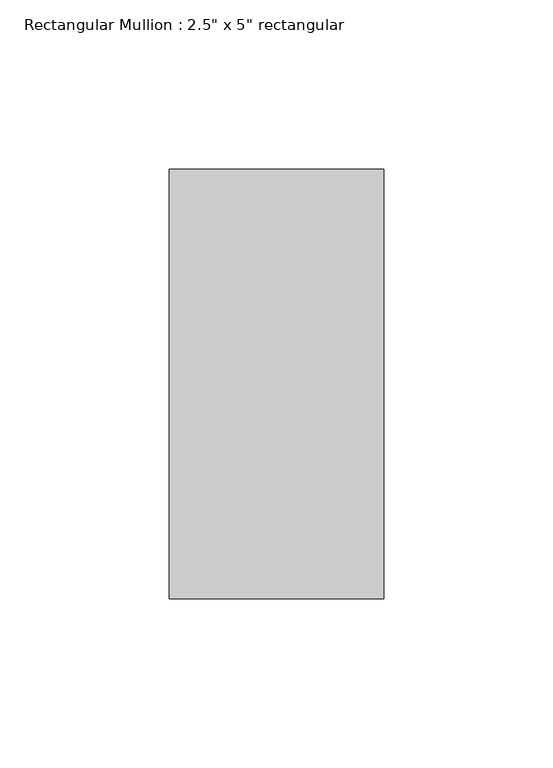
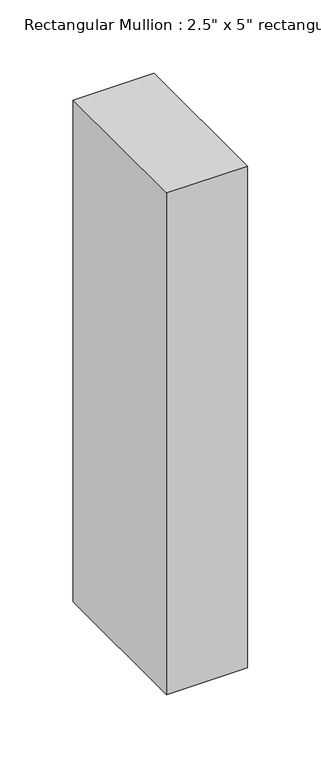
"""IFC4 building model written with IfcOpenShell, lengths in millimetres: member geometry."""

from ifc_helpers import new_model, si_unit, frame, origin, place, context, project, spatial, polyline, outline, extrude, source, transform, mapped, element, save


def member_5a7758d4(model_context):
    return source(origin(), model_context, "Body", "SweptSolid", [
        extrude(outline(polyline([(0.0, 63.5), (0.0, -63.5), (-63.5, -63.5), (-63.5, 63.5), (0.0, 63.5)])), frame((0.0, 0.0, -416.6478549), z_axis=(0.0, 0.0, 1.0), x_axis=(1.0, 0.0, 0.0)), (0.0, 0.0, 1.0), 416.6478549),
    ])


if __name__ == "__main__":
    model = new_model("IFC4")
    model_context = context("Model", 3, world=origin())
    ifc_project = project(units=[si_unit("LENGTHUNIT", "METRE", prefix="MILLI")], contexts=[model_context])
    site = spatial("IfcSite", under=ifc_project)
    building = spatial("IfcBuilding", under=site)
    placement = place(None, origin())
    member_shape = member_5a7758d4(model_context)
    element("IfcMember", 1, ObjectType="Rectangular Mullion : 2.5\" x 5\" rectangular", at=placement, inside=building, context=model_context, shape_type="MappedRepresentation", body=[
        mapped(member_shape, transform((0.0, 0.0, 0.0), x_axis=(1.0, 0.0, 0.0), y_axis=(0.0, 1.0, 0.0), z_axis=(0.0, 0.0, 1.0))),
    ])
    save(model, "model.ifc")

# Revit data of these elements
# Type "Rectangular Mullion : 2.5\" x 5\" rectangular"
#   built-in parameter 1007304 = 0.416667 (stored number, unit not read)
#   built-in parameter 1007301 = 0.104167 (stored number, unit not read)
#   built-in parameter 1007300 = 0.104167 (stored number, unit not read)
# Element 1 (IfcMember, "Rectangular Mullion : 2.5\" x 5\" rectangular")
#   Materials on its faces: "Aluminum"
# Materials
#   "Aluminum": class "Metal", colour RGB 247 247 247, transparency 0, Description = "Aluminum 6061", Cost = 0
